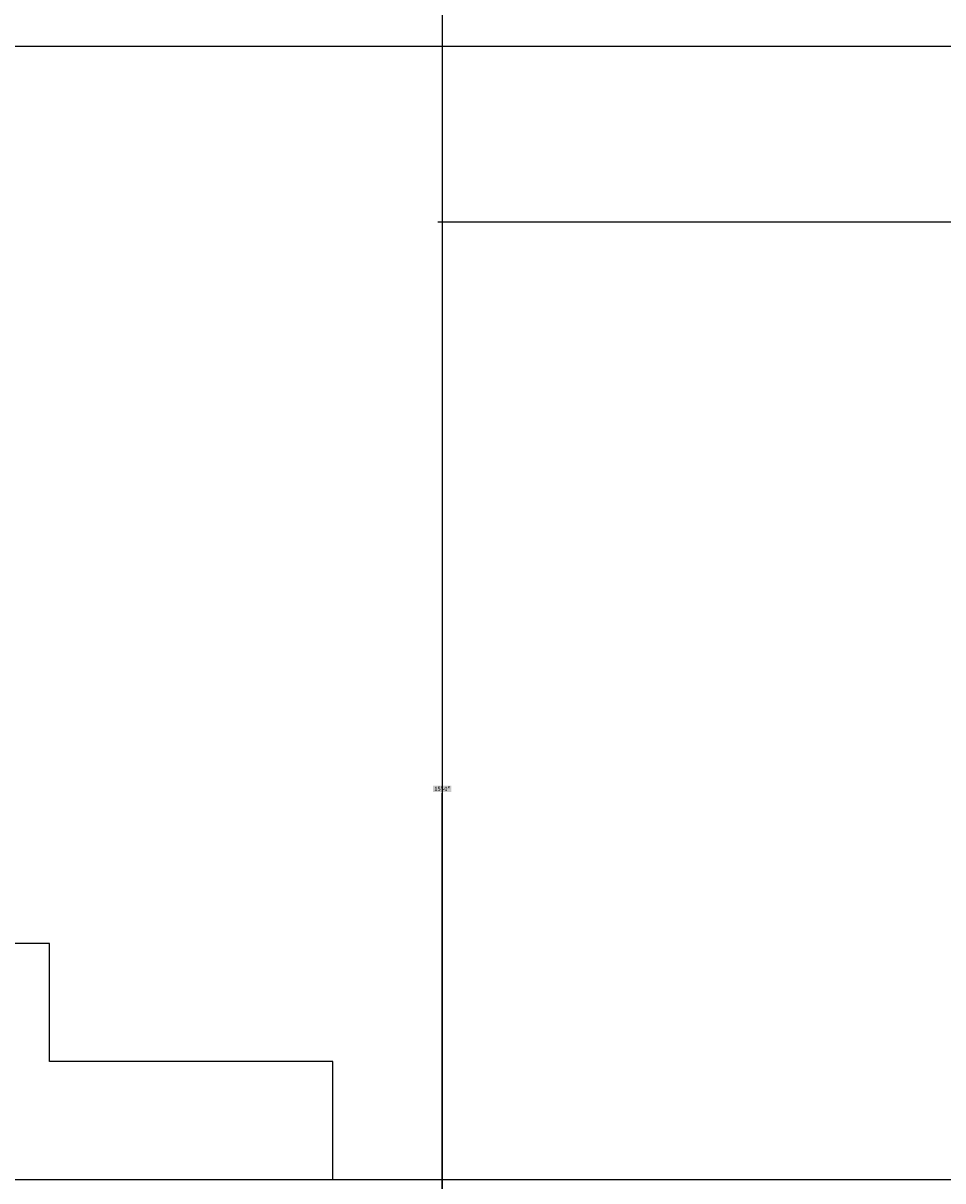
# Model space of a CAD drawing. Units: inches. Extents: x -128 to 854, y -395 to 398.
# Tile 18 of 61: x 329 to 368, y -298 to -249. Entities that reach past the tile are written whole.
import ezdxf

# ---------------------------------------------------------------- set-up
doc = ezdxf.new("R2010")
doc.units = ezdxf.units.IN
doc.header["$MEASUREMENT"] = 0
for name, color, linetype, lineweight in [('A-ANNO-DIMS', 2, 'Continuous', 18), ('A-FLOR-STRS', 7, 'Continuous', 25), ('C-GRAD', 7, 'Continuous', 25)]:
    doc.layers.add(name, color=color, linetype=linetype, lineweight=lineweight)
doc.styles.get("Standard").update_dxf_attribs({"font": 'arial.ttf'})
doc.dimstyles.get("Standard").update_dxf_attribs({"dimtxt": 0.18, "dimasz": 0.18, "dimexe": 0.18, "dimexo": 0.0625, "dimgap": 0.09, "dimtad": 0, "dimtih": 1, "dimtoh": 1, "dimdec": 1, "dimzin": 0, "dimdsep": 46, "dimlunit": 4, "dimtxsty": 'Standard', "dimcen": 0.09, "dimclrd": 1, "dimclre": 2, "dimclrt": 6, "dimadec": 0, "dimazin": 0, "dimtfac": 1, "dimtdec": 1, "dimtofl": 0, "dimtmove": 0, "dimatfit": 3, "dimfxl": 1, "dimtfill": 2, "dimtfillclr": 3, "dimtolj": 1, "dimtzin": 0, "dimarcsym": 0})

# ---------------------------------------------------------------- blocks, each defined once
blk = doc.blocks.new('ENTRY-STEPS-SECTION')
for p, q in [((12, 5), (12, 10)), ((12, 10), (24, 10)), ((0, 0), (0, 5)), ((0, 5), (12, 5)), ((24, 0), (0, 0))]:
    blk.add_line(p, q)
blk = doc.blocks.new('*D120')
at = {"layer": 'A-ANNO-DIMS', "color": 2, "lineweight": -2, "transparency": 16777216}
for p, q in [((317.902, -178.019), (389.719, -178.019)), ((337.902, -358.019), (389.719, -358.019))]:
    blk.add_line(p, q, dxfattribs=at)
at = {"layer": 'A-ANNO-DIMS', "color": 1, "lineweight": -2, "transparency": 16777216}
for p, q in [((389.539, -178.199), (389.539, -267.837)), ((389.539, -357.839), (389.539, -268.201))]:
    blk.add_line(p, q, dxfattribs=at)
at = {"layer": 'A-ANNO-DIMS', "color": 1, "transparency": 16777216}
for points in [[(389.509, -178.199), (389.569, -178.199), (389.539, -178.019)], [(389.509, -357.839), (389.569, -357.839), (389.539, -358.019)]]:
    blk.add_solid(points, dxfattribs=at)
at = {"layer": 'Defpoints', "color": 0, "transparency": 16777216}
for p in [(317.839, -178.019), (337.839, -358.019), (389.539, -358.019)]:
    blk.add_point(p, dxfattribs=at)
at = {"layer": 'A-ANNO-DIMS', "color": 6, "transparency": 16777216, "insert": (389.539, -268.019), "char_height": 0.18, "attachment_point": 5, "bg_fill": 1, "box_fill_scale": 1.25, "bg_fill_color": 3, "bg_fill_transparency": 0}
blk.add_mtext('\\A1;15\'-0"', dxfattribs=at)
blk = doc.blocks.new('*D127')
at = {"layer": 'A-ANNO-DIMS', "color": 2, "lineweight": -2, "transparency": 16777216}
for p, q in [((260.902, -202.019), (389.719, -202.019)), ((317.902, -298.019), (389.719, -298.019))]:
    blk.add_line(p, q, dxfattribs=at)
at = {"layer": 'A-ANNO-DIMS', "color": 1, "lineweight": -2, "transparency": 16777216}
for p, q in [((389.539, -202.199), (389.539, -249.837)), ((389.539, -297.839), (389.539, -250.201))]:
    blk.add_line(p, q, dxfattribs=at)
at = {"layer": 'A-ANNO-DIMS', "color": 1, "transparency": 16777216}
for points in [[(389.509, -202.199), (389.569, -202.199), (389.539, -202.019)], [(389.509, -297.839), (389.569, -297.839), (389.539, -298.019)]]:
    blk.add_solid(points, dxfattribs=at)
at = {"layer": 'Defpoints', "color": 0, "transparency": 16777216}
for p in [(260.839, -202.019), (389.539, -202.019), (317.839, -298.019)]:
    blk.add_point(p, dxfattribs=at)
at = {"layer": 'A-ANNO-DIMS', "color": 6, "transparency": 16777216, "insert": (389.539, -250.019), "char_height": 0.18, "attachment_point": 5, "bg_fill": 1, "box_fill_scale": 1.25, "bg_fill_color": 3, "bg_fill_transparency": 0}
blk.add_mtext('\\A1;8\'-0"', dxfattribs=at)
blk = doc.blocks.new('*D132')
at = {"layer": 'A-ANNO-DIMS', "color": 2, "lineweight": -2, "transparency": 16777216}
for p, q in [((198.902, -250.019), (389.719, -250.019)), ((160.902, -298.019), (389.719, -298.019))]:
    blk.add_line(p, q, dxfattribs=at)
at = {"layer": 'A-ANNO-DIMS', "color": 1, "lineweight": -2, "transparency": 16777216}
for p, q in [((389.539, -250.199), (389.539, -273.837)), ((389.539, -297.839), (389.539, -274.201))]:
    blk.add_line(p, q, dxfattribs=at)
at = {"layer": 'A-ANNO-DIMS', "color": 1, "transparency": 16777216}
for points in [[(389.509, -250.199), (389.569, -250.199), (389.539, -250.019)], [(389.509, -297.839), (389.569, -297.839), (389.539, -298.019)]]:
    blk.add_solid(points, dxfattribs=at)
at = {"layer": 'Defpoints', "color": 0, "transparency": 16777216}
for p in [(198.839, -250.019), (389.539, -250.019), (160.839, -298.019)]:
    blk.add_point(p, dxfattribs=at)
at = {"layer": 'A-ANNO-DIMS', "color": 6, "transparency": 16777216, "insert": (389.539, -274.019), "char_height": 0.18, "attachment_point": 5, "bg_fill": 1, "box_fill_scale": 1.25, "bg_fill_color": 3, "bg_fill_transparency": 0}
blk.add_mtext('\\A1;4\'-0"', dxfattribs=at)
blk = doc.blocks.new('*D134')
at = {"layer": 'A-ANNO-DIMS', "color": 2, "lineweight": -2, "transparency": 16777216}
for p, q in [((418.217, -191.476), (346.3, -191.476)), ((418.217, -371.476), (346.3, -371.476))]:
    blk.add_line(p, q, dxfattribs=at)
at = {"layer": 'A-ANNO-DIMS', "color": 1, "lineweight": -2, "transparency": 16777216}
for p, q in [((346.48, -191.656), (346.48, -281.295)), ((346.48, -371.296), (346.48, -281.658))]:
    blk.add_line(p, q, dxfattribs=at)
at = {"layer": 'A-ANNO-DIMS', "color": 1, "transparency": 16777216}
for points in [[(346.45, -191.656), (346.51, -191.656), (346.48, -191.476)], [(346.45, -371.296), (346.51, -371.296), (346.48, -371.476)]]:
    blk.add_solid(points, dxfattribs=at)
at = {"layer": 'Defpoints', "color": 0, "transparency": 16777216}
for p in [(346.48, -191.476), (418.28, -191.476), (418.28, -371.476)]:
    blk.add_point(p, dxfattribs=at)
at = {"layer": 'A-ANNO-DIMS', "color": 6, "transparency": 16777216, "insert": (346.48, -281.476), "char_height": 0.18, "attachment_point": 5, "bg_fill": 1, "box_fill_scale": 1.25, "bg_fill_color": 3, "bg_fill_transparency": 0}
blk.add_mtext('\\A1;15\'-0"', dxfattribs=at)
blk = doc.blocks.new('*D140')
at = {"layer": 'A-ANNO-DIMS', "color": 2, "lineweight": -2, "transparency": 16777216}
for p, q in [((551.245, -257.476), (346.3, -257.476)), ((551.245, -353.476), (346.3, -353.476))]:
    blk.add_line(p, q, dxfattribs=at)
at = {"layer": 'A-ANNO-DIMS', "color": 1, "lineweight": -2, "transparency": 16777216}
for p, q in [((346.48, -257.656), (346.48, -305.295)), ((346.48, -353.296), (346.48, -305.658))]:
    blk.add_line(p, q, dxfattribs=at)
at = {"layer": 'A-ANNO-DIMS', "color": 1, "transparency": 16777216}
for points in [[(346.45, -257.656), (346.51, -257.656), (346.48, -257.476)], [(346.45, -353.296), (346.51, -353.296), (346.48, -353.476)]]:
    blk.add_solid(points, dxfattribs=at)
at = {"layer": 'Defpoints', "color": 0, "transparency": 16777216}
for p in [(346.48, -257.476), (551.307, -257.476), (551.307, -353.476)]:
    blk.add_point(p, dxfattribs=at)
at = {"layer": 'A-ANNO-DIMS', "color": 6, "transparency": 16777216, "insert": (346.48, -305.476), "char_height": 0.18, "attachment_point": 5, "bg_fill": 1, "box_fill_scale": 1.25, "bg_fill_color": 3, "bg_fill_transparency": 0}
blk.add_mtext('\\A1;8\'-0"', dxfattribs=at)

msp = doc.modelspace()

# ---------------------------------------------------------------- linework, layer by layer
at = {"layer": 'C-GRAD'}
msp.add_line((317.839, -298.019), (365.839, -298.019), dxfattribs=at)

# ---------------------------------------------------------------- block references
at = {"layer": 'A-FLOR-STRS', "extrusion": (0, 0, -1), "zscale": -1}
msp.add_blockref('ENTRY-STEPS-SECTION', (-341.839, -298.019), dxfattribs=at)

# ---------------------------------------------------------------- dimensions: what is measured, and where the dimension line sits
at = {"layer": 'A-ANNO-DIMS'}
for base, p1, p2, picture, middle in [((389.539, -358.019), (317.839, -178.019), (337.839, -358.019), '*D120', (389.539, -268.019)), ((346.48, -191.476), (418.28, -371.476), (418.28, -191.476), '*D134', (346.48, -281.476)), ((389.539, -202.019), (317.839, -298.019), (260.839, -202.019), '*D127', (389.539, -250.019)), ((389.539, -250.019), (160.839, -298.019), (198.839, -250.019), '*D132', (389.539, -274.019)), ((346.48, -257.476), (551.307, -353.476), (551.307, -257.476), '*D140', (346.48, -305.476))]:
    dim = msp.add_linear_dim(base=base, p1=p1, p2=p2, angle=90, dimstyle='Standard', override={"dimdec": 1, "dimlfac": 1, "dimrnd": 0, "dimzin": 1, "dimdsep": 46, "dimlunit": 4, "dimfrac": 2}, dxfattribs=at)
    dim.commit()
    dim.dimension.update_dxf_attribs({"geometry": picture, "text_midpoint": middle})

doc.saveas('drawing.dxf')
